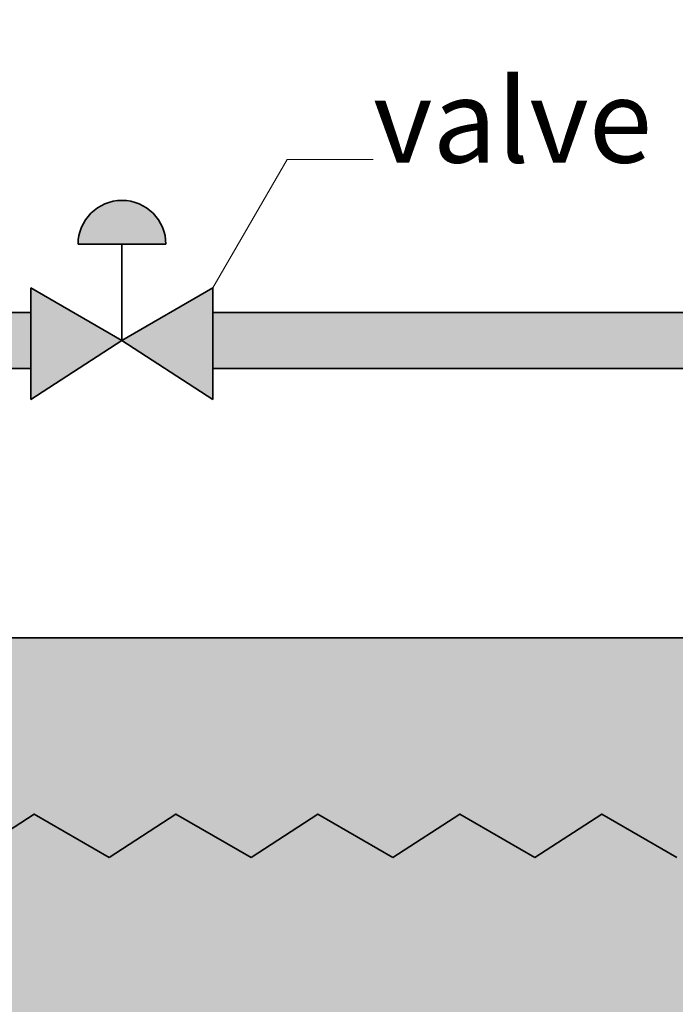
# Model space of a CAD drawing. Units: inches. Extents: x -1 to 292, y -3 to 199.
# Tile 29 of 52: x 123 to 146, y 95 to 130. Entities that reach past the tile are written whole.
import ezdxf

# ---------------------------------------------------------------- set-up
doc = ezdxf.new("R2010")
doc.units = ezdxf.units.IN
doc.header["$MEASUREMENT"] = 0
for name, color, linetype, lineweight in [('M-ANNO-LEAD', 2, 'Continuous', 18), ('M-ANNO-TEXT', 3, 'Continuous', 25), ('M-DIMS', 2, 'Continuous', 18), ('M-EQPM', 7, 'Continuous', 35), ('M-PATT', 8, 'Continuous', 13)]:
    doc.layers.add(name, color=color, linetype=linetype, lineweight=lineweight)
doc.styles.get("Standard").update_dxf_attribs({"font": 'arial.ttf'})
doc.dimstyles.get("Standard").update_dxf_attribs({"dimtxt": 0.18, "dimasz": 0.18, "dimexe": 0.18, "dimexo": 0.0625, "dimgap": 0.09, "dimtad": 0, "dimtih": 1, "dimtoh": 1, "dimdec": 4, "dimzin": 0, "dimdsep": 46, "dimtxsty": 'Standard', "dimcen": 0.09, "dimadec": 0, "dimazin": 0, "dimtfac": 1, "dimtdec": 4, "dimtofl": 0, "dimtmove": 0, "dimatfit": 3, "dimfxl": 1, "dimtolj": 1, "dimtzin": 0, "dimarcsym": 0})

# ---------------------------------------------------------------- blocks, each defined once
blk = doc.blocks.new('*D9')
at = {"layer": 'Defpoints', "color": 0, "transparency": 16777216}
for p in [(177.053, 174.363), (49.924, 99.774), (177.053, 99.774)]:
    blk.add_point(p, dxfattribs=at)
at = {"layer": 'M-DIMS', "color": 0, "lineweight": -2, "transparency": 16777216}
for p, q in [((49.924, 99.836), (49.924, 174.543)), ((50.104, 174.363), (113.033, 174.363)), ((176.873, 174.363), (113.943, 174.363)), ((177.053, 99.836), (177.053, 174.543))]:
    blk.add_line(p, q, dxfattribs=at)
at = {"layer": 'M-DIMS', "color": 0, "transparency": 16777216}
for points in [[(50.104, 174.393), (50.104, 174.333), (49.924, 174.363)], [(176.873, 174.393), (176.873, 174.333), (177.053, 174.363)]]:
    blk.add_solid(points, dxfattribs=at)
at = {"layer": 'M-DIMS', "color": 0, "transparency": 16777216, "insert": (113.488, 174.363), "char_height": 0.18, "attachment_point": 5}
blk.add_mtext('\\A1;127.13', dxfattribs=at)

msp = doc.modelspace()

# ---------------------------------------------------------------- hatches: boundary and pattern name
at = {"layer": 'M-PATT'}
h = msp.add_hatch(color=256, dxfattribs=at)
h.set_gradient(color1=(0, 127, 0), color2=(0, 127, 0), tint=1, name='CYLINDER')
h.paths.add_polyline_path([(164.5186, 119.2985), (129.9293, 119.2985), (129.9293, 117.2985), (164.1897, 117.2985)])
h.paths.add_polyline_path([(181.5897, 119.2985), (164.5186, 119.2985), (164.1897, 117.2985), (179.5897, 117.2985), (179.5897, 107.8518), (181.5897, 109.1506)])
h.paths.add_polyline_path([(181.5897, 109.1506), (179.5897, 107.8518), (179.5897, 36.2698), (198.4159, 36.2698), (198.4159, 38.2698), (181.5897, 38.2698)])
h.paths.add_polyline_path([(115.4883, 126.765), (111.4883, 126.765), (111.4883, 114.6589), (115.4883, 114.6589)])
h.paths.add_polyline_path([(123.408, 119.2985), (115.4883, 119.2985), (115.4883, 117.2985), (123.408, 117.2985)])
h.paths.add_polyline_path([(115.4883, 112.6589), (111.4883, 112.6589), (111.4883, 106.9941), (115.4883, 106.9941)])
h.paths.add_polyline_path([(120.9032, 106.9941), (106.0735, 106.9941), (106.0735, 105.9941), (120.9032, 105.9941)])
h.paths.add_polyline_path([(236.4209, 117.5104), (234.9209, 117.5104), (234.9209, 97.1861), (236.4209, 97.1861)])
h.paths.add_polyline_path([(236.4209, 126.4904), (234.9209, 126.4904), (234.9209, 118.9331), (236.4209, 118.9331)])
h.paths.add_polyline_path([(244.9552, 125.7269), (242.9552, 125.7269), (242.9552, 116.8562), (244.9552, 116.8562)])
h.paths.add_polyline_path([(244.9552, 115.1721), (242.9552, 115.1721), (242.9552, 109.7385), (244.9552, 109.7385)])
h.paths.add_polyline_path([(248.4468, 109.7385), (239.4637, 109.7385), (239.4637, 109.4289), (248.4468, 109.4289)])
h = msp.add_hatch(color=256, dxfattribs=at)
h.set_gradient(color1=(147, 39, 143), color2=(205, 32, 39), tint=1, name='CYLINDER')
h.paths.add_polyline_path([(126.6686, 118.2985), (123.408, 120.181), (123.408, 116.181)])
h.paths.add_polyline_path([(129.9293, 120.181), (126.6686, 118.2985), (129.9293, 116.181)])
h.paths.add_polyline_path([(125.0955, 121.7457), (128.2418, 121.7457, 1)])
h = msp.add_hatch(color=256, dxfattribs=at)
h.set_gradient(color1=(237, 31, 36), color2=(242, 113, 114), tint=1, name='CYLINDER')
h.paths.add_polyline_path([(106.0735, 105.9941), (106.0735, 106.9941), (108.0603, 106.9941), (107.8488, 107.6501), (57.8007, 107.6501, 0.4142136), (49.9241, 99.7735), (52.3176, 101.3278), (55.0097, 99.7735), (57.4032, 101.3278), (60.0953, 99.7735), (62.4888, 101.3278), (65.1809, 99.7735), (67.5744, 101.3278), (70.2665, 99.7735), (72.66, 101.3278), (75.3521, 99.7735), (77.7456, 101.3278), (80.4377, 99.7735), (82.8312, 101.3278), (85.5233, 99.7735), (87.9168, 101.3278), (90.6089, 99.7735), (93.0024, 101.3278), (95.6945, 99.7735), (98.088, 101.3278), (100.7801, 99.7735), (103.1736, 101.3278), (105.8657, 99.7735), (108.2592, 101.3278), (110.9513, 99.7735), (113.3448, 101.3278), (116.0369, 99.7735), (118.4304, 101.3278), (121.1225, 99.7735), (123.516, 101.3278), (126.2082, 99.7735), (128.6016, 101.3278), (131.2938, 99.7735), (133.6872, 101.3278), (136.3794, 99.7735), (138.7728, 101.3278), (141.465, 99.7735), (143.8584, 101.3278), (146.5506, 99.7735), (148.944, 101.3278), (151.6362, 99.7735), (154.0296, 101.3278), (156.7218, 99.7735), (159.1152, 101.3278), (160.6222, 100.4578), (160.6222, 107.6501), (115.4883, 107.6501), (115.4883, 106.9941), (120.9032, 106.9941), (120.9032, 105.9941), (120.9032, 103.3981), (106.0735, 103.3981)])
h.paths.add_polyline_path([(169.176, 107.6501), (162.1623, 107.6501), (162.1623, 100.004), (164.2008, 101.3278), (166.893, 99.7735), (169.2864, 101.3278), (171.9786, 99.7735), (174.372, 101.3278), (177.0526, 99.7802, 0.4139642)])
h.paths.add_polyline_path([(111.4883, 107.6501), (107.8488, 107.6501), (108.0603, 106.9941), (111.4883, 106.9941)], flags=17)
h.paths.add_polyline_path([(61.6788, 91.897), (57.8007, 91.897, -0.1099266), (54.4604, 92.6403), (43.2011, 92.6403), (23.9502, 84.4688), (23.9502, 58.376), (43.2011, 47.2615), (50.9409, 47.2615, -0.2705926), (57.8007, 51.2672), (61.6788, 51.2672)])
h.paths.add_polyline_path([(73.6788, 91.897), (70.6788, 91.897), (70.6788, 51.2672), (73.6788, 51.2672)])
h.paths.add_polyline_path([(79.6788, 91.897), (76.6788, 91.897), (76.6788, 51.2672), (79.6788, 51.2672)])
h.paths.add_polyline_path([(67.6788, 91.897), (64.6788, 91.897), (64.6788, 51.2672), (67.6788, 51.2672)])
h.paths.add_polyline_path([(101.6788, 91.897), (82.6788, 91.897), (82.6788, 51.2672), (101.6788, 51.2672)])
h.paths.add_polyline_path([(107.6788, 91.897), (104.6788, 91.897), (104.6788, 51.2672), (107.6788, 51.2672)])
h.paths.add_polyline_path([(113.6788, 91.897), (110.6788, 91.897), (110.6788, 51.2672), (113.6788, 51.2672)])
h.paths.add_polyline_path([(119.6788, 91.897), (116.6788, 91.897), (116.6788, 51.2672), (119.6788, 51.2672)])
h.paths.add_polyline_path([(141.6788, 91.897), (122.6788, 91.897), (122.6788, 51.2672), (141.6788, 51.2672)])
h.paths.add_polyline_path([(147.6788, 91.897), (144.6788, 91.897), (144.6788, 51.2672), (147.6788, 51.2672)])
h.paths.add_polyline_path([(153.6788, 91.897), (150.6788, 91.897), (150.6788, 51.2672), (153.6788, 51.2672)])
h.paths.add_polyline_path([(159.6788, 91.897), (156.6788, 91.897), (156.6788, 51.2672), (159.6788, 51.2672)])
h.paths.add_polyline_path([(179.5897, 92.6403), (172.5163, 92.6403, -0.1099266), (169.176, 91.897), (162.6788, 91.897), (162.6788, 51.2672), (169.176, 51.2672, -0.2705926), (176.0358, 47.2615), (179.5897, 47.2615)])
h.paths.add_polyline_path([(203.0265, 84.4688), (183.7755, 92.6403), (181.5897, 92.6403), (181.5897, 47.2615), (183.7755, 47.2615), (203.0265, 58.376)])
h.paths.add_polyline_path([(184.4188, 61.52), (200.7224, 61.52), (200.7224, 77.7532), (184.4188, 77.7532)], flags=24)
h = msp.add_hatch(color=256, dxfattribs=at)
h.set_gradient(color1=(0, 255, 255), color2=(0, 255, 255), tint=1)
h.paths.add_polyline_path([(75.3521, 99.7735), (72.66, 101.3278), (70.2665, 99.7735), (67.5744, 101.3278), (65.1809, 99.7735), (62.4888, 101.3278), (60.0953, 99.7735), (57.4032, 101.3278), (55.0097, 99.7735), (52.3176, 101.3278), (49.9241, 99.7735, 0.4142136), (57.8007, 91.897), (61.6788, 91.897), (61.6788, 51.2672), (57.8007, 51.2672, 0.8088808), (54.5813, 36.2021), (65.0947, 51.2672), (64.6788, 51.2672), (64.6788, 91.897), (67.6788, 91.897), (67.6788, 51.2672), (65.0947, 51.2672), (54.5813, 36.2021, 0.1056561), (57.8007, 35.5141), (169.176, 35.5141, 1), (169.176, 51.2672), (162.6788, 51.2672), (162.6788, 91.897), (169.176, 91.897, 0.4144629), (177.0526, 99.7802), (174.372, 101.3278), (171.9786, 99.7735), (169.2864, 101.3278), (166.893, 99.7735), (164.2008, 101.3278), (162.1623, 100.004), (162.1623, 96.1027), (160.6222, 96.1027), (160.6222, 100.4578), (159.1152, 101.3278), (156.7218, 99.7735), (154.0296, 101.3278), (151.6362, 99.7735), (148.944, 101.3278), (146.5506, 99.7735), (143.8584, 101.3278), (141.465, 99.7735), (138.7728, 101.3278), (136.3794, 99.7735), (133.6872, 101.3278), (131.2938, 99.7735), (128.6016, 101.3278), (126.2082, 99.7735), (123.516, 101.3278), (121.1225, 99.7735), (118.4304, 101.3278), (116.0369, 99.7735), (113.3448, 101.3278), (110.9513, 99.7735), (108.2592, 101.3278), (105.8657, 99.7735), (103.1736, 101.3278), (100.7801, 99.7735), (98.088, 101.3278), (95.6945, 99.7735), (93.0024, 101.3278), (90.6089, 99.7735), (87.9168, 101.3278), (85.5233, 99.7735), (82.8312, 101.3278), (80.4377, 99.7735), (77.7456, 101.3278)])
h.paths.add_polyline_path([(79.6788, 91.897), (79.6788, 51.2672), (76.6788, 51.2672), (76.6788, 91.897)], flags=16)
h.paths.add_polyline_path([(73.6788, 91.897), (73.6788, 51.2672), (70.6788, 51.2672), (70.6788, 91.897)], flags=16)
h.paths.add_polyline_path([(82.6788, 91.897), (101.6788, 91.897), (101.6788, 51.2672), (82.6788, 51.2672)], flags=16)
h.paths.add_polyline_path([(104.6788, 91.897), (107.6788, 91.897), (107.6788, 51.2672), (104.6788, 51.2672)], flags=16)
h.paths.add_polyline_path([(110.6788, 91.897), (113.6788, 91.897), (113.6788, 51.2672), (110.6788, 51.2672)], flags=16)
h.paths.add_polyline_path([(116.6788, 91.897), (119.6788, 91.897), (119.6788, 51.2672), (116.6788, 51.2672)], flags=16)
h.paths.add_polyline_path([(122.6788, 91.897), (141.6788, 91.897), (141.6788, 51.2672), (144.6788, 51.2672), (144.6788, 91.897), (147.6788, 91.897), (147.6788, 51.2672), (122.6788, 51.2672)], flags=16)
h.paths.add_polyline_path([(150.6788, 91.897), (153.6788, 91.897), (153.6788, 51.2672), (150.6788, 51.2672)], flags=16)
h.paths.add_polyline_path([(156.6788, 91.897), (159.6788, 91.897), (159.6788, 51.2672), (156.6788, 51.2672)], flags=16)

# ---------------------------------------------------------------- linework, layer by layer
at = {"layer": 'M-ANNO-LEAD'}
for p, q in [((129.9293, 120.181), (132.5837, 124.7787)), ((132.5837, 124.7787), (135.6643, 124.7787))]:
    msp.add_line(p, q, dxfattribs=at)
at = {"layer": 'M-EQPM'}
for p, q in [((125.0955, 121.7457), (128.2418, 121.7457)), ((126.6686, 121.7457), (126.6686, 118.2985)), ((123.408, 120.181), (123.408, 116.181)), ((123.408, 120.181), (126.6686, 118.2985)), ((129.9293, 120.181), (126.6686, 118.2985)), ((129.9293, 120.181), (129.9293, 116.181)), ((126.6686, 118.2985), (126.6686, 119.5738)), ((123.408, 116.181), (126.6686, 118.2985)), ((129.9293, 116.181), (126.6686, 118.2985))]:
    msp.add_line(p, q, dxfattribs=at)
for points in [[(115.4883, 119.2985), (123.408, 119.2985)], [(129.9293, 119.2985), (181.5897, 119.2985), (181.5897, 38.2698)], [(115.4883, 117.2985), (123.408, 117.2985)], [(129.9293, 117.2985), (179.5897, 117.2985), (179.5897, 36.2698)], [(160.6222, 107.6501), (115.4883, 107.6501)], [(121.1225, 99.7735), (123.516, 101.3278), (126.2082, 99.7735)], [(126.2082, 99.7735), (128.6016, 101.3278), (131.2938, 99.7735)], [(131.2938, 99.7735), (133.6872, 101.3278), (136.3794, 99.7735)], [(136.3794, 99.7735), (138.7728, 101.3278), (141.465, 99.7735)], [(141.465, 99.7735), (143.8584, 101.3278), (146.5506, 99.7735)]]:
    msp.add_lwpolyline(points, dxfattribs=at)
msp.add_arc((126.6686, 121.7457), 1.5732, 0, 180, dxfattribs=at)

# ---------------------------------------------------------------- texts
at = {"layer": 'M-ANNO-TEXT', "insert": (135.6643, 127.6725), "char_height": 3, "attachment_point": 1}
msp.add_mtext_dynamic_manual_height_columns('valve', width=47.899539, gutter_width=1, heights=[0], dxfattribs=at)

# ---------------------------------------------------------------- dimensions: what is measured, and where the dimension line sits
at = {"layer": 'M-DIMS'}
dim = msp.add_linear_dim(base=(177.0526, 174.3627), p1=(49.9241, 99.7735), p2=(177.0526, 99.7735), dimstyle='Standard', override={"dimdec": 2, "dimlfac": 1, "dimrnd": 0, "dimzin": 0, "dimdsep": 46, "dimlunit": 2}, dxfattribs=at)
dim.commit()
dim.dimension.update_dxf_attribs({"geometry": '*D9', "text_midpoint": (113.4883, 174.3627)})

doc.saveas('drawing.dxf')
